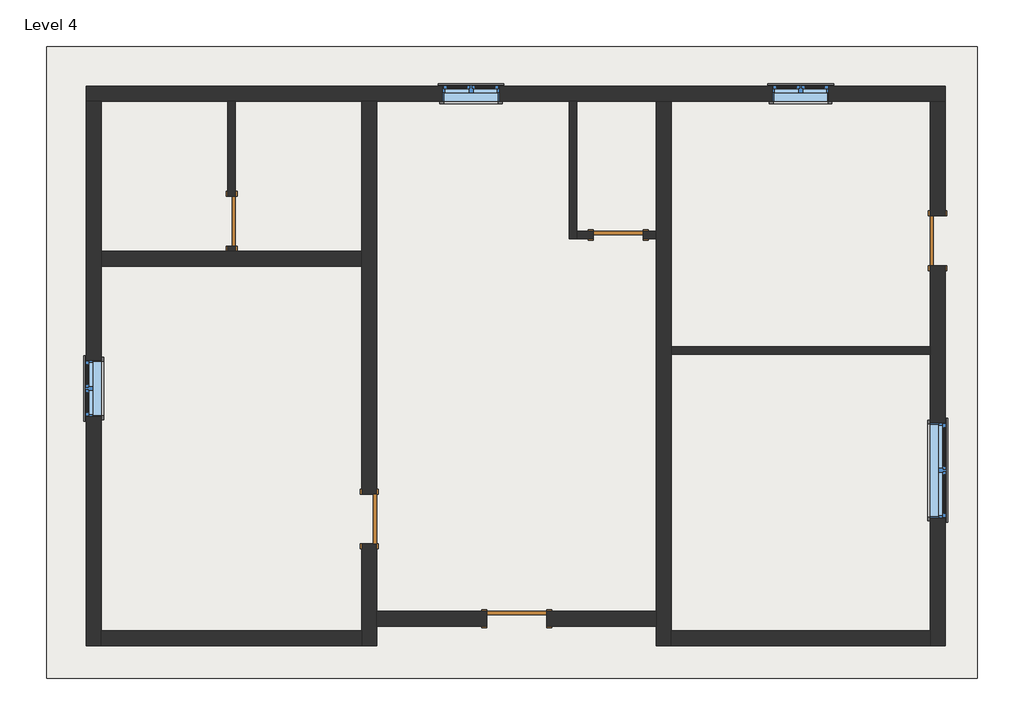
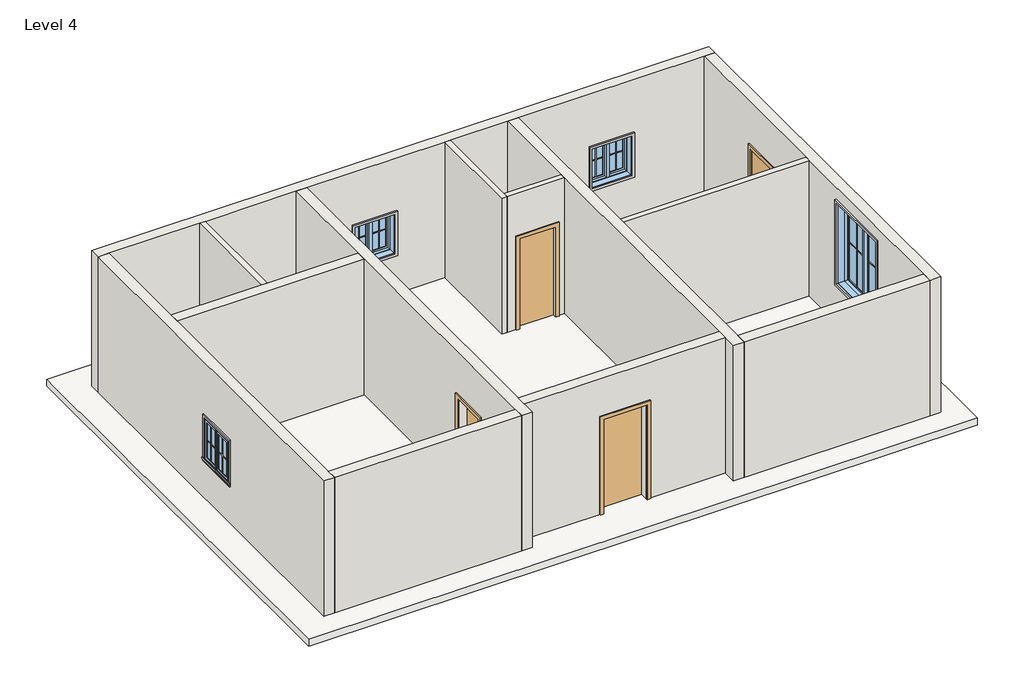
# One storey, incomplete: 16 proxies, 13 walls, 5 doors, 5 windows, 1 roof.
"""IFC4 building model written with IfcOpenShell, lengths in millimetres."""

from ifc_helpers import new_model, si_unit, frame, origin, place, context, project, spatial, polyline, outline, extrude, faceted_brep, transform, mapped, element, save
from components import muntin_pattern_2x2_muntin_pattern_2x2_b3fe6957, muntin_pattern_2x2_muntin_pattern_2x2_3e0ecaf2, muntin_pattern_2x2_muntin_pattern_2x2_bff912c5, muntin_pattern_2x2_muntin_pattern_2x2_c2194282, trim_window_exterior_flat_with_sill_41619996, trim_window_exterior_flat_with_sill_e04b3088, trim_window_interior_flat_picture_frame_51c85655, trim_window_interior_flat_picture_frame_2a7685fe, door_d8f5dbb5, door_f2b275c1, door_85036156, door_0ca8825f, window_aa618e30, window_339605e1, window_9ac97e1a

model = new_model("IFC4")

# Units and contexts
model_context = context("Model", 3, world=origin())
ifc_project = project(units=[si_unit("LENGTHUNIT", "METRE", prefix="MILLI")], contexts=[model_context])

# Site, building, storey
site = spatial("IfcSite", under=ifc_project)
building = spatial("IfcBuilding", under=site)
storey = spatial("IfcBuildingStorey", under=building, Name="Level 4", Elevation=6400.8)

# Proxies
placement = place(None, origin())
muntin_pattern_2x2_muntin_pattern_2x2_shape = muntin_pattern_2x2_muntin_pattern_2x2_b3fe6957(model_context)
element("IfcBuildingElementProxy", 1, Name="Muntin Pattern_2x2 : Muntin Pattern_2x2", ObjectType="Muntin Pattern_2x2 : Muntin Pattern_2x2", at=placement, inside=storey, context=model_context, shape_type="MappedRepresentation", body=[
    mapped(muntin_pattern_2x2_muntin_pattern_2x2_shape, transform((3164.7728376, 7227.4016064, 7385.05), x_axis=(1.0, 0.0, 0.0), y_axis=(0.0, 1.0, 0.0), z_axis=(0.0, 0.0, 1.0))),
])
element("IfcBuildingElementProxy", 2, Name="Muntin Pattern_2x2 : Muntin Pattern_2x2", ObjectType="Muntin Pattern_2x2 : Muntin Pattern_2x2", at=placement, inside=storey, context=model_context, shape_type="MappedRepresentation", body=[
    mapped(muntin_pattern_2x2_muntin_pattern_2x2_shape, transform((-7515.213363, 2411.5985933, 7385.05), x_axis=(0.0, 1.0, 0.0), y_axis=(-1.0, 0.0, 0.0), z_axis=(0.0, 0.0, 1.0))),
])
element("IfcBuildingElementProxy", 3, Name="Muntin Pattern_2x2 : Muntin Pattern_2x2", ObjectType="Muntin Pattern_2x2 : Muntin Pattern_2x2", at=placement, inside=storey, context=model_context, shape_type="MappedRepresentation", body=[
    mapped(muntin_pattern_2x2_muntin_pattern_2x2_shape, transform((-1868.0846872, 7227.4016064, 7385.05), x_axis=(1.0, 0.0, 0.0), y_axis=(0.0, 1.0, 0.0), z_axis=(0.0, 0.0, 1.0))),
])
muntin_pattern_2x2_muntin_pattern_2x2_2_shape = muntin_pattern_2x2_muntin_pattern_2x2_3e0ecaf2(model_context)
element("IfcBuildingElementProxy", 4, Name="Muntin Pattern_2x2 : Muntin Pattern_2x2", ObjectType="Muntin Pattern_2x2 : Muntin Pattern_2x2", at=placement, inside=storey, context=model_context, shape_type="MappedRepresentation", body=[
    mapped(muntin_pattern_2x2_muntin_pattern_2x2_2_shape, transform((3593.3978376, 7227.4016064, 7385.05), x_axis=(-1.0, 0.0, 0.0), y_axis=(0.0, -1.0, 0.0), z_axis=(0.0, 0.0, 1.0))),
])
element("IfcBuildingElementProxy", 5, Name="Muntin Pattern_2x2 : Muntin Pattern_2x2", ObjectType="Muntin Pattern_2x2 : Muntin Pattern_2x2", at=placement, inside=storey, context=model_context, shape_type="MappedRepresentation", body=[
    mapped(muntin_pattern_2x2_muntin_pattern_2x2_2_shape, transform((-7515.213363, 2840.2235933, 7385.05), x_axis=(0.0, -1.0, 0.0), y_axis=(1.0, 0.0, 0.0), z_axis=(0.0, 0.0, 1.0))),
])
element("IfcBuildingElementProxy", 6, Name="Muntin Pattern_2x2 : Muntin Pattern_2x2", ObjectType="Muntin Pattern_2x2 : Muntin Pattern_2x2", at=placement, inside=storey, context=model_context, shape_type="MappedRepresentation", body=[
    mapped(muntin_pattern_2x2_muntin_pattern_2x2_2_shape, transform((-1439.4596872, 7227.4016064, 7385.05), x_axis=(-1.0, 0.0, 0.0), y_axis=(0.0, -1.0, 0.0), z_axis=(0.0, 0.0, 1.0))),
])
muntin_pattern_2x2_muntin_pattern_2x2_3_shape = muntin_pattern_2x2_muntin_pattern_2x2_bff912c5(model_context)
element("IfcBuildingElementProxy", 7, Name="Muntin Pattern_2x2 : Muntin Pattern_2x2", ObjectType="Muntin Pattern_2x2 : Muntin Pattern_2x2", at=placement, inside=storey, context=model_context, shape_type="MappedRepresentation", body=[
    mapped(muntin_pattern_2x2_muntin_pattern_2x2_3_shape, transform((5572.923676, 1735.2928063, 7385.05), x_axis=(0.0, -1.0, 0.0), y_axis=(1.0, 0.0, 0.0), z_axis=(0.0, 0.0, 1.0))),
])
muntin_pattern_2x2_muntin_pattern_2x2_4_shape = muntin_pattern_2x2_muntin_pattern_2x2_c2194282(model_context)
element("IfcBuildingElementProxy", 8, Name="Muntin Pattern_2x2 : Muntin Pattern_2x2", ObjectType="Muntin Pattern_2x2 : Muntin Pattern_2x2", at=placement, inside=storey, context=model_context, shape_type="MappedRepresentation", body=[
    mapped(muntin_pattern_2x2_muntin_pattern_2x2_4_shape, transform((5572.923676, 1014.5678063, 7385.05), x_axis=(0.0, 1.0, 0.0), y_axis=(-1.0, 0.0, 0.0), z_axis=(0.0, 0.0, 1.0))),
])
trim_window_exterior_flat_with_sill_shape = trim_window_exterior_flat_with_sill_41619996(model_context)
element("IfcBuildingElementProxy", 9, Name="Trim-Window-Exterior-Flat : with Sill", ObjectType="Trim-Window-Exterior-Flat : with Sill", at=placement, inside=storey, context=model_context, shape_type="MappedRepresentation", body=[
    mapped(trim_window_exterior_flat_with_sill_shape, transform((3379.0853376, 7236.9266064, 8229.6), x_axis=(-1.0, 0.0, 0.0), y_axis=(0.0, 0.0, 1.0), z_axis=(0.0, 1.0, 0.0))),
])
element("IfcBuildingElementProxy", 10, Name="Trim-Window-Exterior-Flat : with Sill", ObjectType="Trim-Window-Exterior-Flat : with Sill", at=placement, inside=storey, context=model_context, shape_type="MappedRepresentation", body=[
    mapped(trim_window_exterior_flat_with_sill_shape, transform((-7524.738363, 2625.9110933, 8229.6), x_axis=(0.0, -1.0, 0.0), y_axis=(0.0, 0.0, 1.0), z_axis=(-1.0, 0.0, 0.0))),
])
element("IfcBuildingElementProxy", 11, Name="Trim-Window-Exterior-Flat : with Sill", ObjectType="Trim-Window-Exterior-Flat : with Sill", at=placement, inside=storey, context=model_context, shape_type="MappedRepresentation", body=[
    mapped(trim_window_exterior_flat_with_sill_shape, transform((-1653.7721872, 7236.9266064, 8229.6), x_axis=(-1.0, 0.0, 0.0), y_axis=(0.0, 0.0, 1.0), z_axis=(0.0, 1.0, 0.0))),
])
trim_window_exterior_flat_with_sill_2_shape = trim_window_exterior_flat_with_sill_e04b3088(model_context)
element("IfcBuildingElementProxy", 12, Name="Trim-Window-Exterior-Flat : with Sill", ObjectType="Trim-Window-Exterior-Flat : with Sill", at=placement, inside=storey, context=model_context, shape_type="MappedRepresentation", body=[
    mapped(trim_window_exterior_flat_with_sill_2_shape, transform((5582.448676, 1374.9303063, 9144.0), x_axis=(0.0, 1.0, 0.0), y_axis=(0.0, 0.0, 1.0), z_axis=(1.0, 0.0, 0.0))),
])
trim_window_interior_flat_picture_frame_shape = trim_window_interior_flat_picture_frame_51c85655(model_context)
element("IfcBuildingElementProxy", 13, Name="Trim-Window-Interior-Flat : Picture Frame", ObjectType="Trim-Window-Interior-Flat : Picture Frame", at=placement, inside=storey, context=model_context, shape_type="MappedRepresentation", body=[
    mapped(trim_window_interior_flat_picture_frame_shape, transform((3379.0853376, 7008.3266064, 8229.6), x_axis=(1.0, 0.0, 0.0), y_axis=(0.0, 0.0, 1.0), z_axis=(0.0, -1.0, 0.0))),
])
element("IfcBuildingElementProxy", 14, Name="Trim-Window-Interior-Flat : Picture Frame", ObjectType="Trim-Window-Interior-Flat : Picture Frame", at=placement, inside=storey, context=model_context, shape_type="MappedRepresentation", body=[
    mapped(trim_window_interior_flat_picture_frame_shape, transform((-7296.138363, 2625.9110933, 8229.6), x_axis=(0.0, 1.0, 0.0), y_axis=(0.0, 0.0, 1.0), z_axis=(1.0, 0.0, 0.0))),
])
element("IfcBuildingElementProxy", 15, Name="Trim-Window-Interior-Flat : Picture Frame", ObjectType="Trim-Window-Interior-Flat : Picture Frame", at=placement, inside=storey, context=model_context, shape_type="MappedRepresentation", body=[
    mapped(trim_window_interior_flat_picture_frame_shape, transform((-1653.7721872, 7008.3266064, 8229.6), x_axis=(1.0, 0.0, 0.0), y_axis=(0.0, 0.0, 1.0), z_axis=(0.0, -1.0, 0.0))),
])
trim_window_interior_flat_picture_frame_2_shape = trim_window_interior_flat_picture_frame_2a7685fe(model_context)
element("IfcBuildingElementProxy", 16, Name="Trim-Window-Interior-Flat : Picture Frame", ObjectType="Trim-Window-Interior-Flat : Picture Frame", at=placement, inside=storey, context=model_context, shape_type="MappedRepresentation", body=[
    mapped(trim_window_interior_flat_picture_frame_2_shape, transform((5353.848676, 1374.9303063, 9144.0), x_axis=(0.0, -1.0, 0.0), y_axis=(0.0, 0.0, 1.0), z_axis=(-1.0, 0.0, 0.0))),
])

# Doors
door_shape = door_d8f5dbb5(model_context)
element("IfcDoor", 17, ObjectType="Single-Flush : 30\" x 80\"", at=placement, inside=storey, context=model_context, shape_type="MappedRepresentation", body=[
    mapped(door_shape, transform((-5307.8080357, 5179.2254479, 6400.8), x_axis=(0.0, -1.0, 0.0), y_axis=(1.0, 0.0, 0.0), z_axis=(0.0, 0.0, 1.0))),
])
door_2_shape = door_f2b275c1(model_context)
element("IfcDoor", 18, ObjectType="Single-Flush : 30\" x 80\"", at=placement, inside=storey, context=model_context, shape_type="MappedRepresentation", body=[
    mapped(door_2_shape, transform((594.788348, 4969.6493483, 6400.8), x_axis=(-1.0, 0.0, 0.0), y_axis=(0.0, -1.0, 0.0), z_axis=(0.0, 0.0, 1.0))),
])
door_3_shape = door_85036156(model_context)
element("IfcDoor", 19, ObjectType="Single-Flush : 30\" x 80\"", at=placement, inside=storey, context=model_context, shape_type="MappedRepresentation", body=[
    mapped(door_3_shape, transform((5468.148676, 4880.1303063, 6400.8), x_axis=(0.0, -1.0, 0.0), y_axis=(1.0, 0.0, 0.0), z_axis=(0.0, 0.0, 1.0))),
])
element("IfcDoor", 20, ObjectType="Single-Flush : 30\" x 80\"", at=placement, inside=storey, context=model_context, shape_type="MappedRepresentation", body=[
    mapped(door_3_shape, transform((-3207.0990712, 633.8093082, 6400.8), x_axis=(0.0, 1.0, 0.0), y_axis=(-1.0, 0.0, 0.0), z_axis=(0.0, 0.0, 1.0))),
])
door_4_shape = door_0ca8825f(model_context)
element("IfcDoor", 21, ObjectType="Single-Flush : 36\" x 84\"", at=placement, inside=storey, context=model_context, shape_type="MappedRepresentation", body=[
    mapped(door_4_shape, transform((-958.538536, -890.1906918, 6400.8), x_axis=(1.0, 0.0, 0.0), y_axis=(0.0, 1.0, 0.0), z_axis=(0.0, 0.0, 1.0))),
])

# Roof
element("IfcRoof", 22, ObjectType="Generic - 12\"", at=placement, inside=storey, context=model_context, shape_type="SweptSolid", body=[
    extrude(outline(polyline([(-8134.338363, 7846.5266064), (6077.748676, 7846.5266064), (6077.748676, -1794.1868249), (-8134.338363, -1794.1868249), (-8134.338363, 7846.5266064)])), frame((0.0, 0.0, 6248.4), z_axis=(0.0, 0.0, 1.0), x_axis=(1.0, 0.0, 0.0)), (0.0, 0.0, 1.0), 152.4),
])

# Walls
element("IfcWall", 23, ObjectType="WALL4.5\"", at=placement, inside=storey, context=model_context, shape_type="SweptSolid", body=[
    extrude(outline(polyline([(4798.2254479, 8432.8), (4798.2254479, 6400.8), (4722.0254479, 6400.8), (4722.0254479, 9448.8), (7008.3266064, 9448.8), (7008.3266064, 6400.8), (5560.2254479, 6400.8), (5560.2254479, 8432.8), (4798.2254479, 8432.8)])), frame((-5364.9580357, 0.0, 0.0), z_axis=(1.0, 0.0, 0.0), x_axis=(0.0, 1.0, 0.0)), (0.0, 0.0, 1.0), 114.3),
])
element("IfcWall", 24, ObjectType="WALL4.5\"", at=placement, inside=storey, context=model_context, shape_type="Brep", body=[
    faceted_brep([(-157.5953031, 7008.3266064, 6400.8), (-157.5953031, 4912.4993483, 6400.8), (-157.5953031, 4912.4993483, 9448.8), (-157.5953031, 7008.3266064, 9448.8), (-43.2953031, 7008.3266064, 6400.8), (-43.2953031, 7008.3266064, 9448.8), (-43.2953031, 5026.7993483, 9448.8), (-43.2953031, 4912.4993483, 9448.8), (-43.2953031, 4912.4993483, 6400.8), (-43.2953031, 5026.7993483, 6400.8)], [[[0, 1, 2, 3]], [[4, 5, 6, 7, 8, 9]], [[1, 0, 4, 9, 8]], [[0, 3, 5, 4]], [[2, 1, 8, 7]], [[3, 2, 7, 6, 5]]]),
])
element("IfcWall", 25, ObjectType="WALL4.5\"", at=placement, inside=storey, context=model_context, shape_type="SweptSolid", body=[
    extrude(outline(polyline([(6400.8, -43.2953031), (6400.8, 213.788348), (8432.8, 213.788348), (8432.8, 975.788348), (6400.8, 975.788348), (6400.8, 1175.7219991), (9448.8, 1175.7219991), (9448.8, -43.2953031), (6400.8, -43.2953031)])), frame((0.0, 4912.4993483, 0.0), z_axis=(0.0, 1.0, 0.0), x_axis=(0.0, 0.0, 1.0)), (0.0, 0.0, 1.0), 114.3),
])
element("IfcWall", 26, ObjectType="WALL4.5\"", at=placement, inside=storey, context=model_context, shape_type="SweptSolid", body=[
    extrude(outline(polyline([(1404.3219991, 3260.8803063), (5353.848676, 3260.8803063), (5353.848676, 3146.5803063), (1404.3219991, 3146.5803063), (1404.3219991, 3260.8803063)])), frame((0.0, 0.0, 6400.8), z_axis=(0.0, 0.0, 1.0), x_axis=(1.0, 0.0, 0.0)), (0.0, 0.0, 1.0), 3048.0),
])
element("IfcWall", 27, ObjectType="WALL9\"", at=placement, inside=storey, context=model_context, shape_type="Brep", body=[
    faceted_brep([(-7524.738363, 7008.3266064, 6400.8), (-7296.138363, 7008.3266064, 6400.8), (-5364.9580357, 7008.3266064, 6400.8), (-5250.6580357, 7008.3266064, 6400.8), (-3321.3990712, 7008.3266064, 6400.8), (-3092.7990712, 7008.3266064, 6400.8), (-157.5953031, 7008.3266064, 6400.8), (-43.2953031, 7008.3266064, 6400.8), (1175.7219991, 7008.3266064, 6400.8), (1404.3219991, 7008.3266064, 6400.8), (5353.848676, 7008.3266064, 6400.8), (5582.448676, 7008.3266064, 6400.8), (5582.448676, 7008.3266064, 9448.8), (5353.848676, 7008.3266064, 9448.8), (1404.3219991, 7008.3266064, 9448.8), (1175.7219991, 7008.3266064, 9448.8), (-43.2953031, 7008.3266064, 9448.8), (-157.5953031, 7008.3266064, 9448.8), (-3092.7990712, 7008.3266064, 9448.8), (-3321.3990712, 7008.3266064, 9448.8), (-5250.6580357, 7008.3266064, 9448.8), (-5364.9580357, 7008.3266064, 9448.8), (-7296.138363, 7008.3266064, 9448.8), (-7524.738363, 7008.3266064, 9448.8), (-4054.2535534, 7008.3266064, 7188.2), (-4054.2535534, 7008.3266064, 6578.6), (-4460.6535534, 7008.3266064, 6578.6), (-4460.6535534, 7008.3266064, 7188.2), (3810.8853376, 7008.3266064, 8229.6), (3810.8853376, 7008.3266064, 7315.2), (2947.2853376, 7008.3266064, 7315.2), (2947.2853376, 7008.3266064, 8229.6), (-1221.9721872, 7008.3266064, 8229.6), (-1221.9721872, 7008.3266064, 7315.2), (-2085.5721872, 7008.3266064, 7315.2), (-2085.5721872, 7008.3266064, 8229.6), (-7524.738363, 7236.9266064, 6400.8), (-7524.738363, 7236.9266064, 9448.8), (5582.448676, 7236.9266064, 9448.8), (5582.448676, 7236.9266064, 6400.8), (-4054.2535534, 7236.9266064, 7188.2), (-4460.6535534, 7236.9266064, 7188.2), (-4460.6535534, 7236.9266064, 6578.6), (-4054.2535534, 7236.9266064, 6578.6), (3810.8853376, 7236.9266064, 8229.6), (2947.2853376, 7236.9266064, 8229.6), (2947.2853376, 7236.9266064, 7315.2), (3810.8853376, 7236.9266064, 7315.2), (-1221.9721872, 7236.9266064, 8229.6), (-2085.5721872, 7236.9266064, 8229.6), (-2085.5721872, 7236.9266064, 7315.2), (-1221.9721872, 7236.9266064, 7315.2)], [[[0, 1, 2, 3, 4, 5, 6, 7, 8, 9, 10, 11, 12, 13, 14, 15, 16, 17, 18, 19, 20, 21, 22, 23], [24, 25, 26, 27], [28, 29, 30, 31], [32, 33, 34, 35]], [[36, 37, 38, 39], [40, 41, 42, 43], [44, 45, 46, 47], [48, 49, 50, 51]], [[11, 10, 9, 8, 7, 6, 5, 4, 3, 2, 1, 0, 36, 39]], [[12, 11, 39, 38]], [[0, 23, 37, 36]], [[23, 22, 21, 20, 19, 18, 17, 16, 15, 14, 13, 12, 38, 37]], [[25, 24, 40, 43]], [[26, 25, 43, 42]], [[27, 26, 42, 41]], [[24, 27, 41, 40]], [[29, 28, 44, 47]], [[30, 29, 47, 46]], [[31, 30, 46, 45]], [[28, 31, 45, 44]], [[33, 32, 48, 51]], [[34, 33, 51, 50]], [[35, 34, 50, 49]], [[32, 35, 49, 48]]]),
])
element("IfcWall", 28, ObjectType="WALL9\"", at=placement, inside=storey, context=model_context, shape_type="Brep", body=[
    faceted_brep([(5353.848676, 4499.1303063, 8432.8), (5353.848676, 4499.1303063, 6400.8), (5353.848676, 3260.8803063, 6400.8), (5353.848676, 3146.5803063, 6400.8), (5353.848676, -1070.2868249, 6400.8), (5353.848676, -1298.8868249, 6400.8), (5353.848676, -1298.8868249, 9448.8), (5353.848676, -1070.2868249, 9448.8), (5353.848676, 3146.5803063, 9448.8), (5353.848676, 3260.8803063, 9448.8), (5353.848676, 7008.3266064, 9448.8), (5353.848676, 7008.3266064, 6400.8), (5353.848676, 5261.1303063, 6400.8), (5353.848676, 5261.1303063, 8432.8), (5353.848676, 651.0303063, 9144.0), (5353.848676, 651.0303063, 7315.2), (5353.848676, 2098.8303063, 7315.2), (5353.848676, 2098.8303063, 9144.0), (5582.448676, -1298.8868249, 6400.8), (5582.448676, 4499.1303063, 6400.8), (5582.448676, 4499.1303063, 8432.8), (5582.448676, 5261.1303063, 8432.8), (5582.448676, 5261.1303063, 6400.8), (5582.448676, 7008.3266064, 6400.8), (5582.448676, 7008.3266064, 9448.8), (5582.448676, -1298.8868249, 9448.8), (5582.448676, 651.0303063, 9144.0), (5582.448676, 2098.8303063, 9144.0), (5582.448676, 2098.8303063, 7315.2), (5582.448676, 651.0303063, 7315.2)], [[[0, 1, 2, 3, 4, 5, 6, 7, 8, 9, 10, 11, 12, 13], [14, 15, 16, 17]], [[18, 19, 20, 21, 22, 23, 24, 25], [26, 27, 28, 29]], [[12, 11, 23, 22]], [[5, 4, 3, 2, 1, 19, 18]], [[11, 10, 24, 23]], [[6, 5, 18, 25]], [[20, 19, 1, 0]], [[21, 20, 0, 13]], [[22, 21, 13, 12]], [[10, 9, 8, 7, 6, 25, 24]], [[15, 14, 26, 29]], [[16, 15, 29, 28]], [[17, 16, 28, 27]], [[14, 17, 27, 26]]]),
])
element("IfcWall", 29, ObjectType="WALL9\"", at=placement, inside=storey, context=model_context, shape_type="Brep", body=[
    faceted_brep([(-7296.138363, -1298.8868249, 6400.8), (-7296.138363, -1070.2868249, 6400.8), (-7296.138363, 4492.8110933, 6400.8), (-7296.138363, 4721.4110933, 6400.8), (-7296.138363, 7008.3266064, 6400.8), (-7296.138363, 7008.3266064, 9448.8), (-7296.138363, 4721.4110933, 9448.8), (-7296.138363, 4492.8110933, 9448.8), (-7296.138363, -1070.2868249, 9448.8), (-7296.138363, -1298.8868249, 9448.8), (-7296.138363, 3057.7110933, 8229.6), (-7296.138363, 3057.7110933, 7315.2), (-7296.138363, 2194.1110933, 7315.2), (-7296.138363, 2194.1110933, 8229.6), (-7524.738363, -1298.8868249, 6400.8), (-7524.738363, -1298.8868249, 9448.8), (-7524.738363, 7008.3266064, 9448.8), (-7524.738363, 7008.3266064, 6400.8), (-7524.738363, 3057.7110933, 8229.6), (-7524.738363, 2194.1110933, 8229.6), (-7524.738363, 2194.1110933, 7315.2), (-7524.738363, 3057.7110933, 7315.2)], [[[0, 1, 2, 3, 4, 5, 6, 7, 8, 9], [10, 11, 12, 13]], [[14, 15, 16, 17], [18, 19, 20, 21]], [[4, 3, 2, 1, 0, 14, 17]], [[5, 4, 17, 16]], [[0, 9, 15, 14]], [[9, 8, 7, 6, 5, 16, 15]], [[11, 10, 18, 21]], [[12, 11, 21, 20]], [[13, 12, 20, 19]], [[10, 13, 19, 18]]]),
])
element("IfcWall", 30, ObjectType="WALL9\"", at=placement, inside=storey, context=model_context, shape_type="Brep", body=[
    faceted_brep([(-3321.3990712, 7008.3266064, 6400.8), (-3321.3990712, 4721.4110933, 6400.8), (-3321.3990712, 4492.8110933, 6400.8), (-3321.3990712, 1014.8093082, 6400.8), (-3321.3990712, 1014.8093082, 8432.8), (-3321.3990712, 252.8093082, 8432.8), (-3321.3990712, 252.8093082, 6400.8), (-3321.3990712, -1070.2868249, 6400.8), (-3321.3990712, -1298.8868249, 6400.8), (-3321.3990712, -1298.8868249, 9448.8), (-3321.3990712, -1070.2868249, 9448.8), (-3321.3990712, 4492.8110933, 9448.8), (-3321.3990712, 4721.4110933, 9448.8), (-3321.3990712, 7008.3266064, 9448.8), (-3092.7990712, 1014.8093082, 8432.8), (-3092.7990712, 1014.8093082, 6400.8), (-3092.7990712, 7008.3266064, 6400.8), (-3092.7990712, 7008.3266064, 9448.8), (-3092.7990712, -775.8906918, 9448.8), (-3092.7990712, -1004.4906918, 9448.8), (-3092.7990712, -1298.8868249, 9448.8), (-3092.7990712, -1298.8868249, 6400.8), (-3092.7990712, -1004.4906918, 6400.8), (-3092.7990712, -775.8906918, 6400.8), (-3092.7990712, 252.8093082, 6400.8), (-3092.7990712, 252.8093082, 8432.8)], [[[0, 1, 2, 3, 4, 5, 6, 7, 8, 9, 10, 11, 12, 13]], [[14, 15, 16, 17, 18, 19, 20, 21, 22, 23, 24, 25]], [[16, 15, 3, 2, 1, 0]], [[24, 23, 22, 21, 8, 7, 6]], [[0, 13, 17, 16]], [[9, 8, 21, 20]], [[4, 3, 15, 14]], [[5, 4, 14, 25]], [[6, 5, 25, 24]], [[13, 12, 11, 10, 9, 20, 19, 18, 17]]]),
])
element("IfcWall", 31, ObjectType="WALL9\"", at=placement, inside=storey, context=model_context, shape_type="Brep", body=[
    faceted_brep([(1175.7219991, 7008.3266064, 6400.8), (1175.7219991, 5026.7993483, 6400.8), (1175.7219991, 4912.4993483, 6400.8), (1175.7219991, -775.8906918, 6400.8), (1175.7219991, -1004.4906918, 6400.8), (1175.7219991, -1298.8868249, 6400.8), (1175.7219991, -1298.8868249, 9448.8), (1175.7219991, -1004.4906918, 9448.8), (1175.7219991, -775.8906918, 9448.8), (1175.7219991, 4912.4993483, 9448.8), (1175.7219991, 5026.7993483, 9448.8), (1175.7219991, 7008.3266064, 9448.8), (1404.3219991, 7008.3266064, 6400.8), (1404.3219991, 7008.3266064, 9448.8), (1404.3219991, 3260.8803063, 9448.8), (1404.3219991, 3146.5803063, 9448.8), (1404.3219991, -1070.2868249, 9448.8), (1404.3219991, -1298.8868249, 9448.8), (1404.3219991, -1298.8868249, 6400.8), (1404.3219991, -1070.2868249, 6400.8), (1404.3219991, 3146.5803063, 6400.8), (1404.3219991, 3260.8803063, 6400.8)], [[[0, 1, 2, 3, 4, 5, 6, 7, 8, 9, 10, 11]], [[12, 13, 14, 15, 16, 17, 18, 19, 20, 21]], [[5, 4, 3, 2, 1, 0, 12, 21, 20, 19, 18]], [[0, 11, 13, 12]], [[6, 5, 18, 17]], [[11, 10, 9, 8, 7, 6, 17, 16, 15, 14, 13]]]),
])
element("IfcWall", 32, ObjectType="WALL9\"", at=placement, inside=storey, context=model_context, shape_type="SweptSolid", body=[
    extrude(outline(polyline([(-3321.3990712, -1298.8868249), (-7296.138363, -1298.8868249), (-7296.138363, -1070.2868249), (-3321.3990712, -1070.2868249), (-3321.3990712, -1298.8868249)])), frame((0.0, 0.0, 6400.8), z_axis=(0.0, 0.0, 1.0), x_axis=(1.0, 0.0, 0.0)), (0.0, 0.0, 1.0), 3048.0),
])
element("IfcWall", 33, ObjectType="WALL9\"", at=placement, inside=storey, context=model_context, shape_type="SweptSolid", body=[
    extrude(outline(polyline([(5353.848676, -1298.8868249), (1404.3219991, -1298.8868249), (1404.3219991, -1070.2868249), (5353.848676, -1070.2868249), (5353.848676, -1298.8868249)])), frame((0.0, 0.0, 6400.8), z_axis=(0.0, 0.0, 1.0), x_axis=(1.0, 0.0, 0.0)), (0.0, 0.0, 1.0), 3048.0),
])
element("IfcWall", 34, ObjectType="WALL9\"", at=placement, inside=storey, context=model_context, shape_type="SweptSolid", body=[
    extrude(outline(polyline([(8534.4, -501.338536), (6400.8, -501.338536), (6400.8, 1175.7219991), (9448.8, 1175.7219991), (9448.8, -3092.7990712), (6400.8, -3092.7990712), (6400.8, -1415.738536), (8534.4, -1415.738536), (8534.4, -501.338536)])), frame((0.0, -1004.4906918, 0.0), z_axis=(0.0, 1.0, 0.0), x_axis=(0.0, 0.0, 1.0)), (0.0, 0.0, 1.0), 228.6),
])
element("IfcWall", 35, ObjectType="WALL9\"", at=placement, inside=storey, context=model_context, shape_type="SweptSolid", body=[
    extrude(outline(polyline([(-3321.3990712, 4492.8110933), (-7296.138363, 4492.8110933), (-7296.138363, 4721.4110933), (-3321.3990712, 4721.4110933), (-3321.3990712, 4492.8110933)])), frame((0.0, 0.0, 6400.8), z_axis=(0.0, 0.0, 1.0), x_axis=(1.0, 0.0, 0.0)), (0.0, 0.0, 1.0), 3048.0),
])

# Windows
window_shape = window_aa618e30(model_context)
element("IfcWindow", 36, ObjectType="Fixed : 16\" x 24\"", at=placement, inside=storey, context=model_context, shape_type="MappedRepresentation", body=[
    mapped(window_shape, transform((-4219.3535534, 7122.6266064, 5664.2), x_axis=(1.0, 0.0, 0.0), y_axis=(0.0, 1.0, 0.0), z_axis=(0.0, 0.0, 1.0))),
])
window_2_shape = window_339605e1(model_context)
element("IfcWindow", 37, ObjectType="Window-Casement-Double : 34\" x 36\"", at=placement, inside=storey, context=model_context, shape_type="MappedRepresentation", body=[
    mapped(window_2_shape, transform((3379.0853376, 7122.6266064, 6400.8), x_axis=(1.0, 0.0, 0.0), y_axis=(0.0, 1.0, 0.0), z_axis=(0.0, 0.0, 1.0))),
])
element("IfcWindow", 38, ObjectType="Window-Casement-Double : 34\" x 36\"", at=placement, inside=storey, context=model_context, shape_type="MappedRepresentation", body=[
    mapped(window_2_shape, transform((-7410.438363, 2625.9110933, 6400.8), x_axis=(0.0, 1.0, 0.0), y_axis=(-1.0, 0.0, 0.0), z_axis=(0.0, 0.0, 1.0))),
])
element("IfcWindow", 39, ObjectType="Window-Casement-Double : 34\" x 36\"", at=placement, inside=storey, context=model_context, shape_type="MappedRepresentation", body=[
    mapped(window_2_shape, transform((-1653.7721872, 7122.6266064, 6400.8), x_axis=(1.0, 0.0, 0.0), y_axis=(0.0, 1.0, 0.0), z_axis=(0.0, 0.0, 1.0))),
])
window_3_shape = window_9ac97e1a(model_context)
element("IfcWindow", 40, ObjectType="Window-Casement-Double : 57\" x 72\"", at=placement, inside=storey, context=model_context, shape_type="MappedRepresentation", body=[
    mapped(window_3_shape, transform((5468.148676, 1374.9303063, 6400.8), x_axis=(0.0, -1.0, 0.0), y_axis=(1.0, 0.0, 0.0), z_axis=(0.0, 0.0, 1.0))),
])

save(model, "model.ifc")

# Revit data of these elements
# Type "Muntin Pattern_2x2 : Muntin Pattern_2x2"
#   Width [instance default] = 4' - 0"
#   Thickness = 0' - 0 1/2"
#   Height [instance default] = 4' - 0"
#   Distance = 0' - 0 3/4"
#   Interior Material [instance default] = none
#   Exterior Material [instance default] = none
#   Default Elevation = 0
# Type "Trim-Window-Exterior-Flat : with Sill"
#   Trim Width = 0' - 2 1/4"
#   Trim Thickness_Picture Frame = 0' - 1 1/4"
#   Trim Thickness_with Sill = 0' - 0 3/4"
#   Sill Thickness = 0' - 1 1/4"
#   Opening Width [instance default] = 2' - 0"
#   Opening Height [instance default] = 3' - 0"
#   Default Elevation = 4' - 0"
#   Sill = yes
#   Picture Frame = no
#   Trim Material [instance default] = none
# Type "Trim-Window-Interior-Flat : Picture Frame"
#   Trim Thickness_Picture Frame = 0' - 1 1/4"
#   Trim Width = 0' - 2 1/4"
#   Trim Thickness_with Sill = 0' - 0 3/4"
#   Sill Thickness = 0' - 1 1/4"
#   Opening Width [instance default] = 2' - 0"
#   Opening Height [instance default] = 3' - 0"
#   Default Elevation = 4' - 0"
#   Sill = no
#   Picture Frame = yes
#   Trim Material [instance default] = none
# Type "Single-Flush : 30\" x 80\""
#   Type Mark = "5"
#   Construction Type Id = "MDOOR"
#   Assembly Code = "C1020"
#   Analytic Construction = "Metal"
#   Thickness = 0' - 2"
#   Heat Transfer Coefficient (U) = 0.651978 BTU/(h·ft²·°F)
#   Height = 6' - 8"
#   Trim Projection Ext = 0' - 1"
#   Trim Projection Int = 0' - 1"
#   Trim Width = 0' - 3"
#   Width = 2' - 6"
#   Define Thermal Properties by = 1
#   Define Thermal Properties by = 1
#   Door Material = Door - Panel
#   Frame Material = Door - Frame
#   Visual Light Transmittance = 0
#   Solar Heat Gain Coefficient = 0
#   Function = (empty or 0)
#   Wall Closure = (empty or 0)
# Type "Single-Flush : 36\" x 84\""
#   Type Mark = "1"
#   Construction Type Id = "MDOOR"
#   Assembly Code = "C1020"
#   Analytic Construction = "Metal"
#   Thickness = 0' - 2"
#   Heat Transfer Coefficient (U) = 0.651978 BTU/(h·ft²·°F)
#   Height = 7' - 0"
#   Trim Projection Ext = 0' - 1"
#   Trim Projection Int = 0' - 1"
#   Trim Width = 0' - 3"
#   Width = 3' - 0"
#   Define Thermal Properties by = 1
#   Define Thermal Properties by = 1
#   Door Material = Door - Panel
#   Frame Material = Door - Frame
#   Visual Light Transmittance = 0
#   Solar Heat Gain Coefficient = 0
#   Function = (empty or 0)
#   Wall Closure = (empty or 0)
# Type "Generic - 12\""
#   Assembly Code = "B1020"
#   Layers, outside or top first: 0' - 6" no material (function 1)
# Type "WALL4.5\""
#   Assembly Code = "B2010"
#   Layers, outside or top first: 0' - 4 1/2" no material (function 1)
# Type "WALL9\""
#   Assembly Code = "B2010"
#   Layers, outside or top first: 0' - 9" no material (function 1)
# Type "Fixed : 16\" x 24\""
#   Type Mark = "4"
#   Construction Type Id = "GSP4R"
#   Assembly Code = "B2020100"
#   Analytic Construction = "1/8 in Pilkington single glazing"
#   Visual Light Transmittance = 0.9
#   Solar Heat Gain Coefficient = 0.78
#   Heat Transfer Coefficient (U) = 0.6496 BTU/(h·ft²·°F)
#   Height = 2' - 0"
#   Default Sill Height = 3' - 0"
#   Width = 1' - 4"
#   Window Inset = 0' - 0 3/4"
#   Define Thermal Properties by = 1
#   Define Thermal Properties by = 1
#   Glass Pane Material = Glass
#   Sash Material = Sash
#   Wall Closure = (empty or 0)
# Type "Window-Casement-Double : 34\" x 36\""
#   Type Mark = "14"
#   Fire Rating = "0.5h"
#   Assembly Code = "B2020100"
#   Analytic Construction = "Double glazing - domestic"
#   Frame Extension [instance default] = 0' - 0 1/4"
#   Window Inset [instance default] = 0' - 0"
#   Wall Thickness [instance default] = 0' - 6"
#   Interior Wall Closure [instance default] = 0' - 2 1/4"
#   Half Width = 1' - 5"
#   Visual Light Transmittance = 0.81
#   Thermal Resistance (R) = 1.8146 (h·ft²·°F)/BTU
#   Solar Heat Gain Coefficient = 0.76
#   Rough Width = 2' - 10 1/2"
#   Rough Height = 3' - 0 1/2"
#   Height = 3' - 0"
#   Heat Transfer Coefficient (U) = 0.5511 BTU/(h·ft²·°F)
#   Exterior Wall Closure [instance default] = 0' - 1 1/4"
#   Extension Jamb [instance default] = 0' - 2 1/4"
#   Default Sill Height = 3' - 0"
#   Width = 2' - 10"
#   Define Thermal Properties by = 0
#   Muntin Visibility = yes
#   Interior Trim Visibility [instance default] = yes
#   Exterior Trim Visibility [instance default] = yes
#   Extension Jamb Visibility [instance default] = yes
#   Interior Trim Material = Wood - Stained
#   Muntin Pattern = Muntin Pattern_2x2 : Muntin Pattern_2x2
#   Interior Trim = Trim-Window-Interior-Flat : Picture Frame
#   Interior Frame Material = Wood - Stained
#   Glass Panel Material = Glass
#   Exterior Trim Material = Clad - White
#   Exterior Trim = Trim-Window-Exterior-Flat : with Sill
#   Exterior Frame Material = Clad - White
#   Wall Closure = (empty or 0)
# Type "Window-Casement-Double : 57\" x 72\""
#   Type Mark = "17"
#   Fire Rating = "0.5h"
#   Assembly Code = "B2020100"
#   Analytic Construction = "Double glazing - domestic"
#   Frame Extension [instance default] = 0' - 0 1/4"
#   Window Inset [instance default] = 0' - 0"
#   Wall Thickness [instance default] = 0' - 6"
#   Interior Wall Closure [instance default] = 0' - 2 1/4"
#   Half Width = 2' - 4 1/2"
#   Visual Light Transmittance = 0.81
#   Thermal Resistance (R) = 1.8146 (h·ft²·°F)/BTU
#   Solar Heat Gain Coefficient = 0.76
#   Rough Width = 4' - 9 1/2"
#   Rough Height = 6' - 0 1/2"
#   Height = 6' - 0"
#   Heat Transfer Coefficient (U) = 0.5511 BTU/(h·ft²·°F)
#   Exterior Wall Closure [instance default] = 0' - 1 1/4"
#   Extension Jamb [instance default] = 0' - 2 1/4"
#   Default Sill Height = 3' - 0"
#   Width = 4' - 9"
#   Define Thermal Properties by = 0
#   Muntin Visibility = yes
#   Interior Trim Visibility [instance default] = yes
#   Exterior Trim Visibility [instance default] = yes
#   Extension Jamb Visibility [instance default] = yes
#   Interior Trim Material = Wood - Stained
#   Muntin Pattern = Muntin Pattern_2x2 : Muntin Pattern_2x2
#   Interior Trim = Trim-Window-Interior-Flat : Picture Frame
#   Interior Frame Material = Wood - Stained
#   Glass Panel Material = Glass
#   Exterior Trim Material = Clad - White
#   Exterior Trim = Trim-Window-Exterior-Flat : with Sill
#   Exterior Frame Material = Clad - White
#   Wall Closure = (empty or 0)
# Elements 1, 2, 3, 4, 5, 6 (IfcBuildingElementProxy, "Muntin Pattern_2x2 : Muntin Pattern_2x2")
#   Width = 0' - 11 5/8"
#   Height = 2' - 6 1/2"
#   Interior Material = Wood - Stained
#   Exterior Material = Clad - White
#   Phase Created = New Construction
#   Materials on its faces: "Clad - White", "Wood - Stained"
# Elements 7, 8 (IfcBuildingElementProxy, "Muntin Pattern_2x2 : Muntin Pattern_2x2")
#   Width = 1' - 11 1/8"
#   Height = 5' - 6 1/2"
#   Interior Material = Wood - Stained
#   Exterior Material = Clad - White
#   Phase Created = New Construction
#   Materials on its faces: "Clad - White", "Wood - Stained"
# Elements 9, 10, 11 (IfcBuildingElementProxy, "Trim-Window-Exterior-Flat : with Sill")
#   Opening Width = 2' - 10"
#   Opening Height = 3' - 0"
#   Trim Material = Clad - White
#   Phase Created = New Construction
#   Materials on its faces: "Clad - White"
# Element 12 (IfcBuildingElementProxy, "Trim-Window-Exterior-Flat : with Sill")
#   Opening Width = 4' - 9"
#   Opening Height = 6' - 0"
#   Trim Material = Clad - White
#   Phase Created = New Construction
#   Materials on its faces: "Clad - White"
# Elements 13, 14, 15 (IfcBuildingElementProxy, "Trim-Window-Interior-Flat : Picture Frame")
#   Opening Width = 2' - 10"
#   Opening Height = 3' - 0"
#   Trim Material = Wood - Stained
#   Phase Created = New Construction
#   Materials on its faces: "Wood - Stained"
# Element 16 (IfcBuildingElementProxy, "Trim-Window-Interior-Flat : Picture Frame")
#   Opening Width = 4' - 9"
#   Opening Height = 6' - 0"
#   Trim Material = Wood - Stained
#   Phase Created = New Construction
#   Materials on its faces: "Wood - Stained"
# Elements 17, 18, 19, 20 (IfcDoor, "Single-Flush : 30\" x 80\"")
#   Phase Created = New Construction
#   Materials on its faces: "Door - Frame", "Door - Panel"
# Element 21 (IfcDoor, "Single-Flush : 36\" x 84\"")
#   Phase Created = New Construction
#   Materials on its faces: "Door - Frame", "Door - Panel"
# Element 22 (IfcRoof, "Generic - 12\"")
#   built-in parameter 1001705 = 21 (stored number, unit not read)
#   built-in parameter 1001701 = -0.5 (stored number, unit not read)
#   built-in parameter 1001710 = 33615
#   Phase Created = New Construction
#   Materials on its faces: "Default Roof"
# Elements 23, 24, 25, 26 (IfcWall, "WALL4.5\"")
#   Top Offset = 0' - 0"
#   Base Offset = 0' - 0"
#   Unconnected Height = 10' - 0"
#   wall height = 10' - 0"
#   Phase Created = New Construction
#   Base Constraint = Level 4
#   Materials on its faces: "Default Wall"
# Elements 27, 28, 29, 30, 31, 32, 33, 34 (IfcWall, "WALL9\"")
#   Top Offset = 0' - 0"
#   Base Offset = 0' - 0"
#   Unconnected Height = 10' - 0"
#   wall height = 10' - 0"
#   Phase Created = New Construction
#   Base Constraint = Level 4
#   Materials on its faces: "Default Wall", "Blanket"
# Element 35 (IfcWall, "WALL9\"")
#   Top Offset = 0' - 0"
#   Base Offset = 0' - 0"
#   Unconnected Height = 10' - 0"
#   wall height = 10' - 0"
#   Phase Created = New Construction
#   Base Constraint = Level 4
#   Materials on its faces: "Default Wall"
# Element 36 (IfcWindow, "Fixed : 16\" x 24\"")
#   Mark = "11"
#   Phase Created = New Construction
#   Materials on its faces: "Sash", "Glass"
# Element 37 (IfcWindow, "Window-Casement-Double : 34\" x 36\"")
#   Mark = "12"
#   Window Inset = 0' - 0"
#   Interior Wall Closure = 0' - 2 1/4"
#   Frame Extension = 0' - 0 1/4"
#   Exterior Wall Closure = 0' - 1 1/4"
#   Interior Trim Visibility = yes
#   Exterior Trim Visibility = yes
#   Phase Created = New Construction
#   Materials on its faces: "Wood - Stained", "Glass", "Clad - White"
# Element 38 (IfcWindow, "Window-Casement-Double : 34\" x 36\"")
#   Mark = "13"
#   Window Inset = 0' - 0"
#   Interior Wall Closure = 0' - 2 1/4"
#   Frame Extension = 0' - 0 1/4"
#   Exterior Wall Closure = 0' - 1 1/4"
#   Interior Trim Visibility = yes
#   Exterior Trim Visibility = yes
#   Phase Created = New Construction
#   Materials on its faces: "Wood - Stained", "Glass", "Clad - White"
# Element 39 (IfcWindow, "Window-Casement-Double : 34\" x 36\"")
#   Mark = "15"
#   Window Inset = 0' - 0"
#   Interior Wall Closure = 0' - 2 1/4"
#   Frame Extension = 0' - 0 1/4"
#   Exterior Wall Closure = 0' - 1 1/4"
#   Interior Trim Visibility = yes
#   Exterior Trim Visibility = yes
#   Phase Created = New Construction
#   Materials on its faces: "Wood - Stained", "Glass", "Clad - White"
# Element 40 (IfcWindow, "Window-Casement-Double : 57\" x 72\"")
#   Mark = "14"
#   Window Inset = 0' - 0"
#   Interior Wall Closure = 0' - 2 1/4"
#   Frame Extension = 0' - 0 1/4"
#   Exterior Wall Closure = 0' - 1 1/4"
#   Interior Trim Visibility = yes
#   Exterior Trim Visibility = yes
#   Phase Created = New Construction
#   Materials on its faces: "Wood - Stained", "Glass", "Clad - White"
# Materials
#   "Door - Panel": class "Wood", colour RGB 210 159 95, transparency 0, Cost = 0
#   "Door - Frame": colour RGB 118 70 51, transparency 0, Cost = 0
#   "Glass": class "Glass", colour RGB 0 128 192, transparency 0.75, Description = "Soda Lime Glass", Cost = 0
#   "Sash": class "Wood", colour RGB 224 178 126, transparency 0, Cost = 0
#   "Wood - Stained": class "Wood", colour RGB 224 178 126, transparency 0, Cost = 0
#   "Clad - White": class "Wood", colour RGB 242 242 238, transparency 0, Cost = 0
#   "Default Roof": colour RGB 88 101 114, transparency 0, Cost = 0
#   "Default Wall": colour RGB 128 128 128, transparency 0, Cost = 0
#   "Blanket": class "System", colour RGB 59 0 1, transparency 0, Cost = 0
